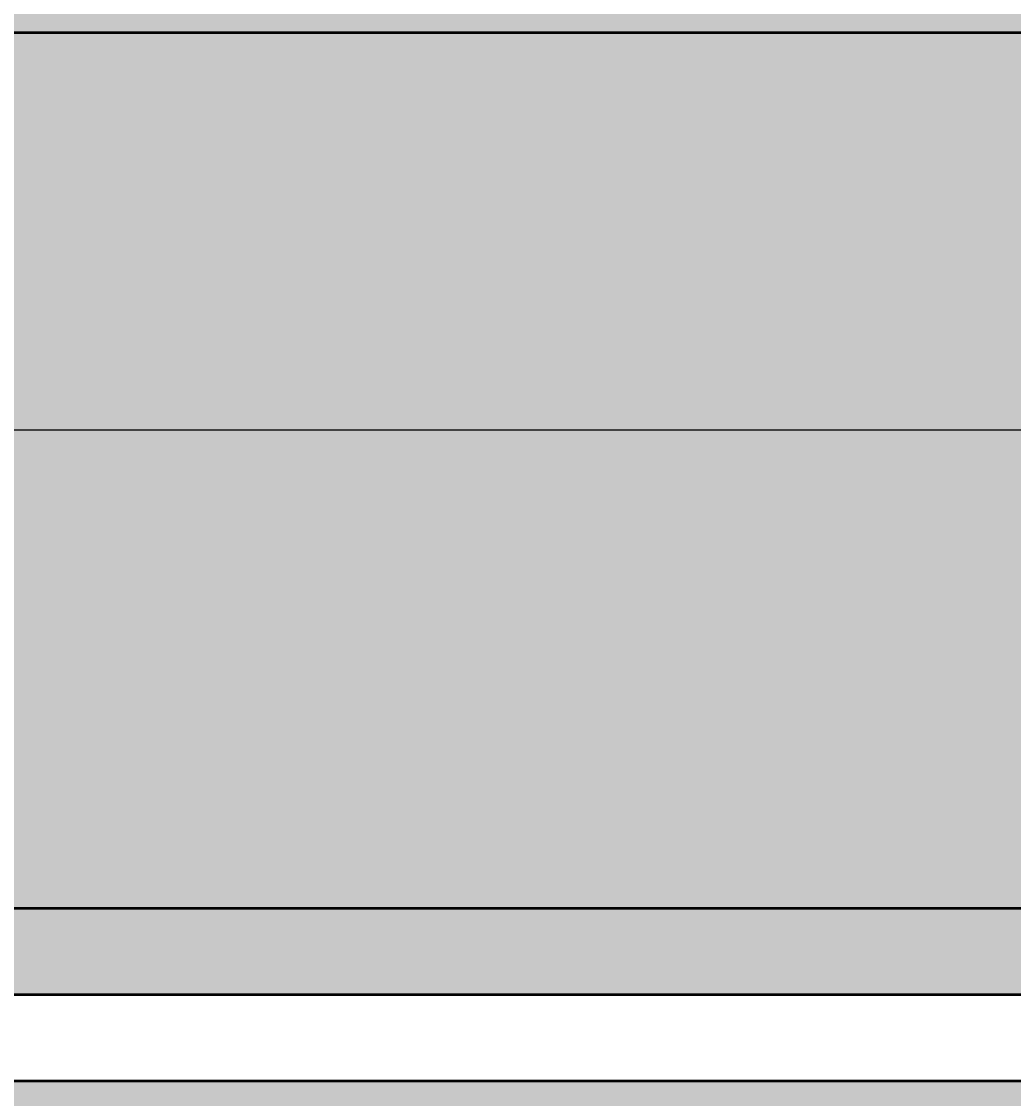
# Model space of a CAD drawing. Units: inches. Extents: x -12 to 334, y -10 to 186.
# Tile 44 of 77: x 175 to 198, y 65 to 90. Entities that reach past the tile are written whole.
import ezdxf

# ---------------------------------------------------------------- set-up
doc = ezdxf.new("R2010")
doc.units = ezdxf.units.IN
doc.header["$MEASUREMENT"] = 0
for name, color, linetype, lineweight in [('M-DIMS', 2, 'Continuous', 18), ('M-EQPM', 7, 'Continuous', 50), ('M-EQPM-PATT', 8, 'Continuous', 18)]:
    doc.layers.add(name, color=color, linetype=linetype, lineweight=lineweight)
doc.styles.get("Standard").update_dxf_attribs({"font": 'arial.ttf'})
doc.dimstyles.get("Standard").update_dxf_attribs({"dimtxt": 0.18, "dimasz": 0.18, "dimexe": 0.18, "dimexo": 0.0625, "dimgap": 0.09, "dimtad": 0, "dimtih": 1, "dimtoh": 1, "dimdec": 4, "dimzin": 0, "dimdsep": 46, "dimtxsty": 'Standard', "dimcen": 0.09, "dimadec": 0, "dimazin": 0, "dimtfac": 1, "dimtdec": 4, "dimtofl": 0, "dimtmove": 0, "dimatfit": 3, "dimfxl": 1, "dimtolj": 1, "dimtzin": 0, "dimarcsym": 0})

# ---------------------------------------------------------------- blocks, each defined once
blk = doc.blocks.new('*D1')
at = {"layer": 'Defpoints', "color": 0, "transparency": 16777216}
for p in [(281.426, 91.899), (3.376, 80.692), (281.426, 14.304)]:
    blk.add_point(p, dxfattribs=at)
at = {"layer": 'M-DIMS', "color": 0, "lineweight": -2, "transparency": 16777216}
for p, q in [((281.426, 91.836), (281.426, 14.124)), ((3.376, 80.629), (3.376, 14.124)), ((3.556, 14.304), (141.935, 14.304)), ((281.246, 14.304), (142.867, 14.304))]:
    blk.add_line(p, q, dxfattribs=at)
at = {"layer": 'M-DIMS', "color": 0, "transparency": 16777216}
for points in [[(3.556, 14.334), (3.556, 14.274), (3.376, 14.304)], [(281.246, 14.334), (281.246, 14.274), (281.426, 14.304)]]:
    blk.add_solid(points, dxfattribs=at)
at = {"layer": 'M-DIMS', "color": 0, "transparency": 16777216, "insert": (142.401, 14.304), "char_height": 0.18, "attachment_point": 5}
blk.add_mtext('\\A1;278.05', dxfattribs=at)
blk = doc.blocks.new('*D17')
at = {"layer": 'Defpoints', "color": 0, "transparency": 16777216}
for p in [(106.177, 102.896), (105.892, 56.321), (295.976, 56.321)]:
    blk.add_point(p, dxfattribs=at)
at = {"layer": 'M-DIMS', "color": 0, "lineweight": -2, "transparency": 16777216}
for p, q in [((106.24, 102.896), (296.156, 102.896)), ((295.976, 102.716), (295.976, 79.79)), ((295.976, 56.501), (295.976, 79.426)), ((105.954, 56.321), (296.156, 56.321))]:
    blk.add_line(p, q, dxfattribs=at)
at = {"layer": 'M-DIMS', "color": 0, "transparency": 16777216}
for points in [[(295.946, 102.716), (296.006, 102.716), (295.976, 102.896)], [(295.946, 56.501), (296.006, 56.501), (295.976, 56.321)]]:
    blk.add_solid(points, dxfattribs=at)
at = {"layer": 'M-DIMS', "color": 0, "transparency": 16777216, "insert": (295.976, 79.608), "char_height": 0.18, "attachment_point": 5}
blk.add_mtext('\\A1;46.575', dxfattribs=at)
blk = doc.blocks.new('*D35')
at = {"layer": 'Defpoints', "color": 0, "transparency": 16777216}
for p in [(216.428, 98.108), (-11.174, 61.105), (216.428, 61.105)]:
    blk.add_point(p, dxfattribs=at)
at = {"layer": 'M-DIMS', "color": 0, "lineweight": -2, "transparency": 16777216}
for p, q in [((216.365, 98.108), (-11.354, 98.108)), ((-11.174, 97.928), (-11.174, 79.788)), ((-11.174, 61.285), (-11.174, 79.424)), ((216.365, 61.105), (-11.354, 61.105))]:
    blk.add_line(p, q, dxfattribs=at)
at = {"layer": 'M-DIMS', "color": 0, "transparency": 16777216}
for points in [[(-11.204, 97.928), (-11.144, 97.928), (-11.174, 98.108)], [(-11.204, 61.285), (-11.144, 61.285), (-11.174, 61.105)]]:
    blk.add_solid(points, dxfattribs=at)
at = {"layer": 'M-DIMS', "color": 0, "transparency": 16777216, "insert": (-11.174, 79.606), "char_height": 0.18, "attachment_point": 5}
blk.add_mtext('\\A1;37', dxfattribs=at)
blk = doc.blocks.new('*D39')
at = {"layer": 'Defpoints', "color": 0, "transparency": 16777216}
for p in [(279.726, 80.692), (-11.174, 45.854), (269.381, 45.854)]:
    blk.add_point(p, dxfattribs=at)
at = {"layer": 'M-DIMS', "color": 0, "lineweight": -2, "transparency": 16777216}
for p, q in [((279.664, 80.692), (-11.354, 80.692)), ((-11.174, 80.512), (-11.174, 63.455)), ((-11.174, 46.034), (-11.174, 63.091)), ((269.318, 45.854), (-11.354, 45.854))]:
    blk.add_line(p, q, dxfattribs=at)
at = {"layer": 'M-DIMS', "color": 0, "transparency": 16777216}
for points in [[(-11.204, 80.512), (-11.144, 80.512), (-11.174, 80.692)], [(-11.204, 46.034), (-11.144, 46.034), (-11.174, 45.854)]]:
    blk.add_solid(points, dxfattribs=at)
at = {"layer": 'M-DIMS', "color": 0, "transparency": 16777216, "insert": (-11.174, 63.273), "char_height": 0.18, "attachment_point": 5}
blk.add_mtext('\\A1;34.84', dxfattribs=at)
blk = doc.blocks.new('*D41')
at = {"layer": 'Defpoints', "color": 0, "transparency": 16777216}
for p in [(190.169, 91.899), (277.343, 68.515)]:
    blk.add_point(p, dxfattribs=at)
at = {"layer": 'M-DIMS', "color": 0, "lineweight": -2, "transparency": 16777216}
for p, q in [((190.079, 91.899), (190.259, 91.899)), ((190.169, 91.809), (190.169, 91.989)), ((329.648, 54.485), (277.517, 68.469)), ((329.828, 54.485), (329.648, 54.485))]:
    blk.add_line(p, q, dxfattribs=at)
at = {"layer": 'M-DIMS', "color": 0, "transparency": 16777216}
blk.add_solid([(277.525, 68.498), (277.509, 68.44), (277.343, 68.515)], dxfattribs=at)
at = {"layer": 'M-DIMS', "color": 0, "transparency": 16777216, "insert": (330.307, 54.485), "char_height": 0.18, "attachment_point": 5}
blk.add_mtext('\\A1;R90.26', dxfattribs=at)

msp = doc.modelspace()

# ---------------------------------------------------------------- hatches: boundary and pattern name
at = {"layer": 'M-EQPM-PATT'}
h = msp.add_hatch(color=256, dxfattribs=at)
h.set_gradient(color1=(205, 32, 39), color2=(205, 32, 39), tint=1)
h.paths.add_polyline_path([(64.5, 80.754), (64.5, 89.8963), (226.6083, 89.8963, -1), (226.6083, 69.6117), (64.5, 69.6117), (64.5, 78.754), (4.4744, 78.754, 0.384914), (23.5807, 61.4872), (37.1002, 61.4872), (37.1002, 33.6752), (53.1002, 33.6752), (53.1002, 61.4872), (64.5, 61.4872), (64.5, 63.6117), (226.6083, 63.6117, 1), (226.6083, 95.8963), (64.5, 95.8963), (64.5, 99.8958), (53.1002, 99.8958), (53.1002, 127.7078), (37.1002, 127.7078), (37.1002, 99.8958), (23.5807, 99.8958, 0.4132606), (4.3766, 80.754)])
h.paths.add_polyline_path([(64.5, 91.8963), (64.5, 93.8963), (226.6083, 93.8963, -1), (226.6083, 65.6117), (64.5, 65.6117), (64.5, 67.6117), (226.6083, 67.6117, 1), (226.6083, 91.8963)], flags=16)
h = msp.add_hatch(color=256, dxfattribs=at)
h.set_gradient(color1=(94, 103, 175), color2=(94, 103, 175), tint=1)
h.paths.add_polyline_path([(129.093, 89.8963), (86.8879, 89.8963), (86.8879, 69.6117), (129.093, 69.6117)], flags=17)
h.paths.add_polyline_path([(170.9079, 89.8963), (130.8573, 89.8963), (130.8573, 69.6117), (170.9079, 69.6117)], flags=17)
h.paths.add_polyline_path([(216.4278, 89.8963), (172.6722, 89.8963), (172.6722, 69.6117), (216.4278, 69.6117)], flags=17)
h.paths.add_polyline_path([(245.9354, 82.6969), (247.9354, 82.6969), (247.9354, 46.8541), (268.3808, 46.8541, 0.0998398), (279.7263, 80.6915), (251.9801, 80.6915, 0.4142136), (231.7758, 100.8958), (84.7229, 100.8958), (84.7229, 109.0583), (83.7229, 109.0583), (83.7229, 95.8963), (129.093, 95.8963), (129.093, 98.1081), (130.8573, 98.1081), (130.8573, 95.8963), (170.9079, 95.8963), (170.9079, 98.1081), (172.6722, 98.1081), (172.6722, 95.8963), (216.4278, 95.8963), (216.4278, 98.1081), (218.1922, 98.1081), (218.1922, 95.8963), (226.6083, 95.8963, -1), (226.6083, 63.6117), (218.1922, 63.6117), (218.1922, 61.1045), (216.4278, 61.1045), (216.4278, 63.6117), (172.6722, 63.6117), (172.6722, 61.1045), (170.9079, 61.1045), (170.9079, 63.6117), (130.8573, 63.6117), (130.8573, 61.1045), (129.093, 61.1045), (129.093, 63.6117), (87.8879, 63.6117), (87.8879, 56.3205), (105.8919, 56.3205), (105.8919, 28.8541), (115.8919, 28.8541), (115.8919, 46.8541), (222.5761, 46.8541), (222.5761, 30.8541), (232.5761, 30.8541), (232.5761, 46.8541), (245.9354, 46.8541)])
h.paths.add_polyline_path([(86.8879, 89.8963), (75.9244, 89.8963), (75.9244, 69.6117), (86.8879, 69.6117)])
h.paths.add_polyline_path([(83.7229, 109.0583), (75.9244, 109.0583), (75.9244, 95.8963), (83.7229, 95.8963)])
h.paths.add_polyline_path([(226.6083, 89.8963), (218.1922, 89.8963), (218.1922, 69.6117), (226.6083, 69.6117, 1)], flags=17)

# ---------------------------------------------------------------- linework, layer by layer
at = {"layer": 'M-EQPM'}
for points in [[(64.5, 65.6117), (226.6083, 65.6117, 1), (226.6083, 93.8963), (64.5, 93.8963)], [(64.5, 67.6117), (226.6083, 67.6117, 1), (226.6083, 91.8963), (64.5, 91.8963)], [(64.5, 69.6117), (226.6083, 69.6117, 1), (226.6083, 89.8963), (64.5, 89.8963)]]:
    msp.add_lwpolyline(points, format="xyb", dxfattribs=at)

# ---------------------------------------------------------------- dimensions: what is measured, and where the dimension line sits
at = {"layer": 'M-DIMS'}
for base, p1, p2, override, picture, middle in [((295.9756, 56.3205), (106.1771, 102.8958), (105.8919, 56.3205), {"dimdec": 3, "dimlfac": 1, "dimrnd": 0, "dimzin": 0, "dimdsep": 46, "dimlunit": 2}, '*D17', (295.9756, 79.6082)), ((-11.1736, 61.1045), (216.4278, 98.1081), (216.4278, 61.1045), {"dimdec": 0, "dimlfac": 1, "dimrnd": 0, "dimzin": 0, "dimdsep": 46, "dimlunit": 2}, '*D35', (-11.1735, 79.6063)), ((-11.1736, 45.8541), (279.7263, 80.6915), (269.3808, 45.8541), {"dimdec": 2, "dimlfac": 1, "dimrnd": 0, "dimzin": 0, "dimdsep": 46, "dimlunit": 2}, '*D39', (-11.1735, 63.2728))]:
    dim = msp.add_linear_dim(base=base, p1=p1, p2=p2, angle=90, dimstyle='Standard', override=override, dxfattribs=at)
    dim.commit()
    dim.dimension.update_dxf_attribs({"geometry": picture, "text_midpoint": middle})
dim = msp.add_linear_dim(base=(281.4256, 14.3041), p1=(3.3765, 80.6915), p2=(281.4256, 91.8988), dimstyle='Standard', override={"dimdec": 2, "dimlfac": 1, "dimrnd": 0, "dimzin": 0, "dimdsep": 46, "dimlunit": 2}, dxfattribs=at)
dim.commit()
dim.dimension.update_dxf_attribs({"geometry": '*D1', "text_midpoint": (142.401, 14.3041)})
dim = msp.add_radius_dim(center=(190.1689, 91.8988), mpoint=(277.3431, 68.5153), dimstyle='Standard', override={"dimdec": 2, "dimlfac": 1, "dimrnd": 0, "dimzin": 0, "dimdsep": 46, "dimlunit": 2}, dxfattribs=at)
dim.commit()
dim.dimension.update_dxf_attribs({"geometry": '*D41', "text_midpoint": (330.3074, 54.4851), "dimtype": 164})

doc.saveas('drawing.dxf')
